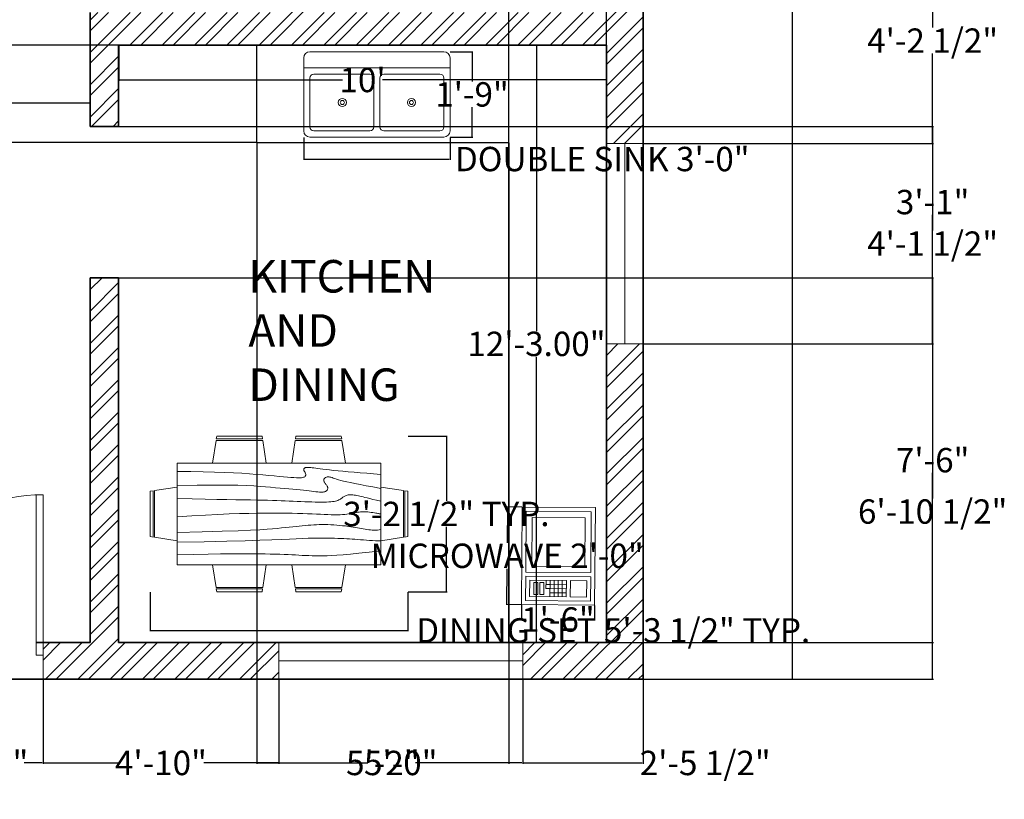
# Model space of a CAD drawing. Units: inches. Extents: x -20 to 887, y -143 to 410.
# Tile 2 of 5: x 139 to 381, y -11 to 180. Entities that reach past the tile are written whole.
import ezdxf

# ---------------------------------------------------------------- set-up
doc = ezdxf.new("R2010")
doc.units = ezdxf.units.IN
doc.header["$MEASUREMENT"] = 0
for name, color, linetype, lineweight in [('A-ANNO-DIMS', 2, 'Continuous', 18), ('A-AREA-IDEN', 7, 'Continuous', 25), ('A-DOOR', 3, 'Continuous', 18), ('A-EQPM', 9, 'Continuous', 18), ('A-FLOR-CASE', 9, 'Continuous', 25), ('A-FLOR-FIXT', 9, 'Continuous', 18), ('A-FURN', 8, 'Continuous', 18), ('A-GLAZ', 4, 'Continuous', 18), ('A-WALL', 7, 'Continuous', 35), ('A-WALL-PATT', 8, 'Continuous', 13)]:
    doc.layers.add(name, color=color, linetype=linetype, lineweight=lineweight)
doc.styles.get("Standard").update_dxf_attribs({"font": 'arial.ttf'})
doc.dimstyles.get("Standard").update_dxf_attribs({"dimtxt": 6, "dimasz": 0.18, "dimexe": 0.18, "dimexo": 0.0625, "dimgap": 0.09, "dimtad": 0, "dimtih": 1, "dimtoh": 1, "dimzin": 0, "dimdsep": 46, "dimlunit": 3, "dimtxsty": 'Standard', "dimcen": 0.09, "dimadec": 0, "dimazin": 0, "dimtfac": 1, "dimtofl": 0, "dimtmove": 0, "dimatfit": 3, "dimfxl": 1, "dimtolj": 1, "dimtzin": 0, "dimarcsym": 0})

# ---------------------------------------------------------------- blocks, each defined once
blk = doc.blocks.new('*U2')
for p, q in [((0, 0), (0, -6)), ((40, 0), (40, -6))]:
    blk.add_line(p, q)
blk.add_lwpolyline([(0, 0), (0, 40), (1.75, 40), (1.75, 0)], close=True)
blk.add_arc((0, 0), 40, 0, 90)
blk = doc.blocks.new('Microwave')
for p, q in [((18, 10), (22, 10)), ((19, 7), (19, 11)), ((20, 11), (20, 7)), ((21, 7), (21, 11)), ((22, 9), (18, 9)), ((18, 8), (22, 8)), ((22, 7), (18, 7)), ((20, 6), (18, 6)), ((19, 6), (19, 7)), ((20, 7), (20, 6))]:
    blk.add_line(p, q)
for points in [[(0, 0), (0, 18), (24, 18), (24, 0)], [(1, 1), (1, 17), (16, 17), (16, 1)], [(17, 1), (17, 17), (23, 17), (23, 1)], [(2.5, 2.5), (2.5, 15.5), (14.5, 15.5), (14.5, 2.5)], [(18, 12), (18, 16), (22, 16), (22, 12)], [(18, 2), (18, 11), (22, 11), (22, 2)], [(18.5, 4.5), (18.5, 5.5), (21.5, 5.5), (21.5, 4.5)], [(18.5, 3), (18.5, 4), (21.5, 4), (21.5, 3)]]:
    blk.add_lwpolyline(points, close=True)
blk = doc.blocks.new('Sink-double - 36 in top')
for p, q in [((-18, -4), (18, -4)), ((-0.75, -18.5), (-0.75, -6.5)), ((0.75, -6.5), (0.75, -18.5))]:
    blk.add_line(p, q)
for points in [[(-16.5, 0), (16.5, 0)], [(-18, -19.5), (-18, -1.5)], [(18, -1.5), (18, -19.5)], [(-16.5, -18.5), (-16.5, -6.5)], [(-15.5, -5.5), (-1.75, -5.5)], [(1.75, -5.5), (15.5, -5.5)], [(16.5, -6.5), (16.5, -18.5)], [(16.5, -21), (-16.5, -21)], [(-1.75, -19.5), (-15.5, -19.5)], [(15.5, -19.5), (1.75, -19.5)]]:
    blk.add_lwpolyline(points)
for centre, radius in [((-8.5, -12.5), 1), ((-8.5, -12.5), 0.5), ((8.5, -12.5), 1), ((8.5, -12.5), 0.5)]:
    blk.add_circle(centre, radius)
for centre, radius, start, end in [((-16.5, -1.5), 1.5, 90, 180), ((16.5, -1.5), 1.5, 0, 90), ((-15.5, -6.5), 1, 90, 180), ((-1.75, -6.5), 1, 0, 90), ((1.75, -6.5), 1, 90, 180), ((15.5, -6.5), 1, 0, 90), ((-15.5, -18.5), 1, 180, 270), ((-1.75, -18.5), 1, 270, 0), ((1.75, -18.5), 1, 180, 270), ((15.5, -18.5), 1, 270, 0), ((-16.5, -19.5), 1.5, 180, 270), ((16.5, -19.5), 1.5, 270, 0)]:
    blk.add_arc(centre, radius, start, end)
blk = doc.blocks.new('Dining Set - 36 x 72 in.')
for p, q in [((-22.2343, 26.00059), (-23.4847, 17.99762)), ((-22.2304, 26), (-5.7608, 26)), ((-22, 27.5), (-22.1562, 26.50042)), ((-5.8416, 26.5), (-22.1534, 26.5)), ((-22, 27.5), (-6, 27.5)), ((-5.8437, 26.49966), (-6, 27.5)), ((-4.5152, 17.99762), (-5.7655, 25.99926)), ((5.7657, 26.00059), (4.5153, 17.99762)), ((5.7696, 26), (22.2392, 26)), ((6, 27.5), (5.8438, 26.50042)), ((22.1584, 26.5), (5.8466, 26.5)), ((6, 27.5), (22, 27.5)), ((22.1563, 26.49966), (22, 27.5)), ((23.4848, 17.99762), (22.2345, 25.99926)), ((36, 18), (-36, 18)), ((-36, 18), (-36, -18)), ((36, -18), (36, 18)), ((-45.5, 8), (-44.5004, 8.15617)), ((-45.5, 8), (-45.5, -8)), ((-44.5, -8.15843), (-44.5, 8.15338)), ((-44.0006, 8.23428), (-35.9976, 9.48474)), ((-44, 8.23041), (-44, -8.23915)), ((44.0006, 8.23428), (35.9976, 9.48474)), ((44, 8.23041), (44, -8.23915)), ((44.5, -8.15843), (44.5, 8.15338)), ((45.5, 8), (44.5005, 8.15617)), ((45.5, 8), (45.5, -8)), ((-44.4997, -8.15631), (-45.5, -8)), ((-35.9976, -9.48476), (-43.9993, -8.2345)), ((35.9976, -9.48476), (43.9993, -8.2345)), ((44.4997, -8.15631), (45.5, -8)), ((-36, -18), (36, -18)), ((-22.2343, -26.0006), (-23.4847, -17.99762)), ((-4.5152, -17.99762), (-5.7655, -25.99928)), ((5.7657, -26.0006), (4.5153, -17.99762)), ((23.4848, -17.99762), (22.2345, -25.99928)), ((-22.2304, -26), (-5.7608, -26)), ((-22, -27.5), (-22.1562, -26.50044)), ((-5.8416, -26.5), (-22.1534, -26.5)), ((-22, -27.5), (-6, -27.5)), ((-5.8437, -26.49967), (-6, -27.5)), ((5.7696, -26), (22.2392, -26)), ((6, -27.5), (5.8438, -26.50044)), ((22.1584, -26.5), (5.8466, -26.5)), ((6, -27.5), (22, -27.5)), ((22.1563, -26.49967), (22, -27.5))]:
    blk.add_line(p, q)
for points in [[(-36, 15), (-31.1772, 14.97754), (-26.8079, 14.91406), (-22.8538, 14.81543), (-19.276, 14.6875), (-16.0362, 14.53613), (-13.0957, 14.36718), (-10.4159, 14.18652), (-7.9583, 14), (-5.6904, 13.81315), (-3.6035, 13.63021), (-1.6954, 13.45508), (0.0365, 13.29166), (1.5945, 13.14388), (2.9811, 13.01562), (4.1988, 12.9108), (5.25, 12.83333), (6.1393, 12.78613), (6.8802, 12.76823), (7.4883, 12.77767), (7.9792, 12.8125), (8.3685, 12.87077), (8.6719, 12.95052), (8.9049, 13.0498), (9.0833, 13.16666), (9.2205, 13.29899), (9.3216, 13.44401), (9.3895, 13.59879), (9.4271, 13.76041), (9.4373, 13.92594), (9.4232, 14.09245), (9.3875, 14.257), (9.3333, 14.41666), (9.2638, 14.56917), (9.1836, 14.71484), (9.0975, 14.85465), (9.0104, 14.98958), (8.9272, 15.1206), (8.8529, 15.2487), (8.7922, 15.37483), (8.75, 15.5), (8.7305, 15.62467), (8.7344, 15.74739), (8.7617, 15.86621), (8.8125, 15.97916), (8.8867, 16.08431), (8.9844, 16.17968), (9.1055, 16.26334), (9.25, 16.33333), (9.4189, 16.38802), (9.6172, 16.42708), (9.8506, 16.45052), (10.125, 16.45833), (10.4463, 16.45052), (10.8203, 16.42708), (11.2529, 16.38802), (11.75, 16.33333), (12.3184, 16.26318), (12.9694, 16.17838), (13.7151, 16.07991), (14.5677, 15.96875), (15.5395, 15.84586), (16.6426, 15.71224), (17.8893, 15.56884), (19.2917, 15.41666), (20.859, 15.25667), (22.5879, 15.08984), (24.4721, 14.91715), (26.5052, 14.73958), (28.6809, 14.5581), (30.9929, 14.3737), (33.4347, 14.18733), (36, 14)], [(-36, 10), (-28.9766, 10.14274), (-23.1725, 10.20442), (-18.4241, 10.19775), (-14.5677, 10.13541), (-11.4399, 10.03011), (-8.877, 9.89453), (-6.7154, 9.74137), (-4.7917, 9.58333), (-2.9698, 9.43082), (-1.2246, 9.28515), (0.4415, 9.14534), (2.026, 9.01041), (3.5266, 8.87939), (4.9408, 8.7513), (6.266, 8.62516), (7.5, 8.5), (8.6411, 8.37549), (9.6914, 8.2539), (10.6538, 8.13818), (11.5312, 8.03125), (12.3267, 7.93603), (13.043, 7.85547), (13.6831, 7.79248), (14.25, 7.75), (14.7471, 7.7303), (15.1797, 7.73307), (15.5537, 7.75732), (15.875, 7.80208), (16.1494, 7.86637), (16.3828, 7.94922), (16.5811, 8.04964), (16.75, 8.16666), (16.8944, 8.29915), (17.0143, 8.44531), (17.1089, 8.60319), (17.1771, 8.77083), (17.218, 8.94629), (17.2305, 9.1276), (17.2137, 9.31282), (17.1667, 9.5), (17.0895, 9.6875), (16.987, 9.875), (16.8649, 10.0625), (16.7292, 10.25), (16.5856, 10.4375), (16.4401, 10.625), (16.2985, 10.8125), (16.1667, 11), (16.05, 11.18733), (15.9518, 11.3737), (15.8752, 11.5581), (15.8229, 11.73958), (15.798, 11.91715), (15.8034, 12.08984), (15.842, 12.25667), (15.9167, 12.41666), (16.0295, 12.56836), (16.1784, 12.70833), (16.3605, 12.83268), (16.5729, 12.9375), (16.8127, 13.01888), (17.0768, 13.07291), (17.3625, 13.0957), (17.6667, 13.08333), (17.9894, 13.03312), (18.3418, 12.94726), (18.7382, 12.82918), (19.1927, 12.68229), (19.7195, 12.51001), (20.3327, 12.31575), (21.0465, 12.10294), (21.875, 11.875), (22.8357, 11.63354), (23.959, 11.37304), (25.2786, 11.08618), (26.8282, 10.76562), (28.6414, 10.40405), (30.752, 9.99414), (33.1936, 9.52856), (36, 9)], [(-36, 5.5), (-30.7157, 5.3348), (-26.069, 5.20963), (-21.9946, 5.11767), (-18.4271, 5.05208), (-15.3009, 5.00602), (-12.5508, 4.97265), (-10.1112, 4.94515), (-7.9167, 4.91666), (-5.909, 4.88167), (-4.0586, 4.83984), (-2.3429, 4.79215), (-0.7396, 4.73958), (0.7739, 4.6831), (2.22, 4.6237), (3.6213, 4.56233), (5, 4.5), (6.373, 4.43782), (7.7344, 4.3776), (9.0723, 4.32129), (10.375, 4.27083), (11.6309, 4.22819), (12.8281, 4.19531), (13.9551, 4.17415), (15, 4.16666), (15.954, 4.17448), (16.819, 4.19791), (17.6001, 4.23698), (18.3021, 4.29166), (18.9299, 4.36198), (19.4883, 4.44791), (19.9823, 4.54948), (20.4167, 4.66666), (20.7969, 4.79899), (21.1302, 4.94401), (21.4245, 5.09879), (21.6875, 5.26041), (21.9271, 5.42594), (22.1511, 5.59245), (22.3672, 5.757), (22.5834, 5.91666), (22.8065, 6.06868), (23.0404, 6.21093), (23.2879, 6.34147), (23.5521, 6.45833), (23.8358, 6.55957), (24.142, 6.64323), (24.4735, 6.70735), (24.8334, 6.75), (25.2235, 6.76969), (25.642, 6.76692), (26.0858, 6.74267), (26.5521, 6.69791), (27.0379, 6.63362), (27.5404, 6.55078), (28.0565, 6.45036), (28.5834, 6.33333), (29.1242, 6.19987), (29.7071, 6.04687), (30.3661, 5.87044), (31.1354, 5.66666), (32.0493, 5.43164), (33.142, 5.16146), (34.4475, 4.85221), (36, 4.5)], [(-36, -1), (-30.7915, -0.6591), (-26.0195, -0.38216), (-21.6519, -0.16284), (-17.6563, 0.00521), (-14.0005, 0.12833), (-10.6523, 0.21289), (-7.5796, 0.26522), (-4.75, 0.29166), (-2.134, 0.29793), (0.2878, 0.28711), (2.5317, 0.26163), (4.6146, 0.22396), (6.5529, 0.17651), (8.3633, 0.12174), (10.0623, 0.06209), (11.6667, 0), (13.1899, -0.06201), (14.6341, -0.1211), (15.9982, -0.17432), (17.2813, -0.21875), (18.4823, -0.25147), (19.6003, -0.26953), (20.6343, -0.27002), (21.5834, -0.25), (22.4481, -0.20768), (23.2357, -0.14584), (23.9549, -0.06836), (24.6146, 0.02083), (25.2235, 0.11784), (25.7904, 0.21875), (26.3241, 0.31966), (26.8334, 0.41666), (27.3265, 0.50618), (27.8099, 0.58593), (28.2894, 0.65397), (28.7709, 0.70833), (29.2601, 0.74707), (29.763, 0.76823), (30.2855, 0.76985), (30.8334, 0.75), (31.4088, 0.70784), (31.9994, 0.64713), (32.589, 0.57275), (33.1615, 0.48958), (33.7008, 0.4025), (34.1908, 0.3164), (34.6153, 0.23616), (34.9584, 0.16666), (35.2099, 0.11165), (35.3848, 0.07031), (35.504, 0.04069), (35.5886, 0.02083), (35.6594, 0.00879), (35.7377, 0.0026), (35.8442, 0.00032), (36, 0)], [(-36, -6.5), (-27.1843, -6.31267), (-20.084, -6.1263), (-14.469, -5.9419), (-10.1094, -5.76042), (-6.7752, -5.58285), (-4.2363, -5.41016), (-2.2629, -5.24333), (-0.625, -5.08334), (0.8708, -4.93099), (2.2715, -4.78646), (3.5872, -4.64974), (4.8281, -4.52084), (6.0046, -4.39974), (7.127, -4.28646), (8.2053, -4.18099), (9.25, -4.08334), (10.2705, -3.99382), (11.2734, -3.91407), (12.2647, -3.84603), (13.25, -3.79167), (14.2354, -3.75293), (15.2266, -3.73177), (16.2295, -3.73015), (17.25, -3.75), (18.2912, -3.79248), (19.3451, -3.85547), (20.4009, -3.93604), (21.4479, -4.03125), (22.4754, -4.13819), (23.4727, -4.25391), (24.4289, -4.37549), (25.3334, -4.5), (26.1785, -4.62492), (26.9694, -4.74935), (27.7145, -4.87281), (28.4219, -4.99479), (29.1, -5.11483), (29.7572, -5.23242), (30.4016, -5.34709), (31.0417, -5.45834), (31.6837, -5.56437), (32.3262, -5.65821), (32.9658, -5.73153), (33.599, -5.77604), (34.2224, -5.78345), (34.8327, -5.74545), (35.4264, -5.65373), (36, -5.5)], [(-36, -10), (-26.4022, -9.81299), (-18.4675, -9.62891), (-11.9839, -9.45069), (-6.7396, -9.28125), (-2.5226, -9.12354), (0.8789, -8.98047), (3.6769, -8.85498), (6.0833, -8.75), (8.2767, -8.66765), (10.3021, -8.60677), (12.1712, -8.56543), (13.8958, -8.54167), (15.4876, -8.53353), (16.9583, -8.53907), (18.3197, -8.55632), (19.5834, -8.58334), (20.7616, -8.61841), (21.8685, -8.66081), (22.9188, -8.71004), (23.9271, -8.76563), (24.9081, -8.82707), (25.8763, -8.89388), (26.8465, -8.96558), (27.8334, -9.04167), (28.8474, -9.12118), (29.8828, -9.20117), (30.93, -9.27824), (31.9792, -9.34896), (33.0205, -9.40991), (34.0443, -9.45768), (35.0407, -9.48885), (36, -9.5)], [(-36, -14.5), (-30.0881, -14.33513), (-25.0332, -14.21224), (-20.7312, -14.12647), (-17.0781, -14.07292), (-13.97, -14.04671), (-11.3027, -14.04297), (-8.9724, -14.05681), (-6.875, -14.08334), (-4.9224, -14.11833), (-3.0905, -14.16016), (-1.3709, -14.20785), (0.2448, -14.26042), (1.7647, -14.3169), (3.1973, -14.3763), (4.5507, -14.43767), (5.8333, -14.5), (7.0554, -14.5621), (8.235, -14.62175), (9.3922, -14.67652), (10.5469, -14.72396), (11.7192, -14.76164), (12.929, -14.78711), (14.1965, -14.79794), (15.5417, -14.79167), (16.9933, -14.76424), (18.6152, -14.70508), (20.4804, -14.60197), (22.6615, -14.44271), (25.2312, -14.21509), (28.2624, -13.9069), (31.8277, -13.50594), (36, -13)]]:
    blk.add_lwpolyline(points)
blk = doc.blocks.new('*D12')
at = {"layer": 'A-ANNO-DIMS', "color": 0, "lineweight": -2, "transparency": 16777216}
for p, q in [((25.42, 164.4), (25.42, 159.66)), ((156.42, 164.4), (156.42, 159.66)), ((25.6, 159.84), (72.65, 159.84)), ((156.24, 159.84), (109.19, 159.84))]:
    blk.add_line(p, q, dxfattribs=at)
at = {"layer": 'A-ANNO-DIMS', "color": 0, "transparency": 16777216}
for points in [[(25.6, 159.87), (25.6, 159.81), (25.42, 159.84)], [(156.24, 159.87), (156.24, 159.81), (156.42, 159.84)]]:
    blk.add_solid(points, dxfattribs=at)
at = {"layer": 'Defpoints', "color": 0, "transparency": 16777216}
for p in [(25.42, 164.46), (156.42, 164.46), (156.42, 159.84)]:
    blk.add_point(p, dxfattribs=at)
at = {"layer": 'A-ANNO-DIMS', "color": 0, "transparency": 16777216, "insert": (90.92, 159.84), "char_height": 6, "attachment_point": 5}
blk.add_mtext('\\A1;10\'-11.00"', dxfattribs=at)
blk = doc.blocks.new('*D13')
at = {"layer": 'A-ANNO-DIMS', "color": 0, "lineweight": -2, "transparency": 16777216}
for p, q in [((163.42, 174.07), (163.42, 165.37)), ((283.42, 174.07), (283.42, 165.37)), ((163.6, 165.55), (218.52, 165.55)), ((283.24, 165.55), (228.32, 165.55))]:
    blk.add_line(p, q, dxfattribs=at)
at = {"layer": 'A-ANNO-DIMS', "color": 0, "transparency": 16777216}
for points in [[(163.6, 165.58), (163.6, 165.52), (163.42, 165.55)], [(283.24, 165.58), (283.24, 165.52), (283.42, 165.55)]]:
    blk.add_solid(points, dxfattribs=at)
at = {"layer": 'Defpoints', "color": 0, "transparency": 16777216}
for p in [(163.42, 174.13), (283.42, 174.13), (283.42, 165.55)]:
    blk.add_point(p, dxfattribs=at)
at = {"layer": 'A-ANNO-DIMS', "color": 0, "transparency": 16777216, "insert": (223.42, 165.55), "char_height": 6, "attachment_point": 5}
blk.add_mtext("\\A1;10'", dxfattribs=at)
blk = doc.blocks.new('*D14')
at = {"layer": 'A-ANNO-DIMS', "color": 0, "lineweight": -2, "transparency": 16777216}
for p, q in [((283.35, 174.13), (266.02, 174.13)), ((266.2, 173.95), (266.2, 103.79)), ((266.2, 27.31), (266.2, 97.48)), ((283.35, 27.13), (266.02, 27.13))]:
    blk.add_line(p, q, dxfattribs=at)
at = {"layer": 'A-ANNO-DIMS', "color": 0, "transparency": 16777216}
for points in [[(266.17, 173.95), (266.23, 173.95), (266.2, 174.13)], [(266.17, 27.31), (266.23, 27.31), (266.2, 27.13)]]:
    blk.add_solid(points, dxfattribs=at)
at = {"layer": 'Defpoints', "color": 0, "transparency": 16777216}
for p in [(266.2, 174.13), (283.42, 174.13), (283.42, 27.13)]:
    blk.add_point(p, dxfattribs=at)
at = {"layer": 'A-ANNO-DIMS', "color": 0, "transparency": 16777216, "insert": (266.2, 100.63), "char_height": 6, "attachment_point": 5}
blk.add_mtext('\\A1;12\'-3.00"', dxfattribs=at)
blk = doc.blocks.new('*D22')
at = {"layer": 'A-ANNO-DIMS', "color": 0, "lineweight": -2, "transparency": 16777216}
for p, q in [((292.48, 378.13), (329.35, 378.13)), ((329.17, 377.95), (329.17, 201.29)), ((329.17, 18.31), (329.17, 194.98)), ((292.48, 18.13), (329.35, 18.13))]:
    blk.add_line(p, q, dxfattribs=at)
at = {"layer": 'A-ANNO-DIMS', "color": 0, "transparency": 16777216}
for points in [[(329.14, 377.95), (329.2, 377.95), (329.17, 378.13)], [(329.14, 18.31), (329.2, 18.31), (329.17, 18.13)]]:
    blk.add_solid(points, dxfattribs=at)
at = {"layer": 'Defpoints', "color": 0, "transparency": 16777216}
for p in [(292.42, 378.13), (292.42, 18.13), (329.17, 18.13)]:
    blk.add_point(p, dxfattribs=at)
at = {"layer": 'A-ANNO-DIMS', "color": 0, "transparency": 16777216, "insert": (329.17, 198.13), "char_height": 6, "attachment_point": 5}
blk.add_mtext("\\A1;30'", dxfattribs=at)
blk = doc.blocks.new('*D47')
at = {"layer": 'A-ANNO-DIMS', "color": 0, "lineweight": -2, "transparency": 16777216}
for p, q in [((171.19, 39.58), (171.19, 29.96)), ((234.54, 39.58), (234.54, 29.96)), ((171.37, 30.14), (234.36, 30.14)), ((234.54, 30.14), (234.72, 30.14))]:
    blk.add_line(p, q, dxfattribs=at)
at = {"layer": 'A-ANNO-DIMS', "color": 0, "transparency": 16777216}
for points in [[(171.37, 30.17), (171.37, 30.11), (171.19, 30.14)], [(234.36, 30.17), (234.36, 30.11), (234.54, 30.14)]]:
    blk.add_solid(points, dxfattribs=at)
at = {"layer": 'Defpoints', "color": 0, "transparency": 16777216}
for p in [(171.19, 39.64), (234.54, 39.64), (234.54, 30.14)]:
    blk.add_point(p, dxfattribs=at)
at = {"layer": 'A-ANNO-DIMS', "color": 0, "transparency": 16777216, "insert": (285.08, 30.14), "char_height": 6, "attachment_point": 5}
blk.add_mtext('\\A1;DINING SET 5\'-3 1/2" TYP.', dxfattribs=at)
blk = doc.blocks.new('*D48')
at = {"layer": 'A-ANNO-DIMS', "color": 0, "lineweight": -2, "transparency": 16777216}
for p, q in [((234.6, 77.93), (244.22, 77.93)), ((244.04, 77.75), (244.04, 61.98)), ((244.04, 39.82), (244.04, 55.59)), ((234.6, 39.64), (244.22, 39.64))]:
    blk.add_line(p, q, dxfattribs=at)
at = {"layer": 'A-ANNO-DIMS', "color": 0, "transparency": 16777216}
for points in [[(244.01, 77.75), (244.07, 77.75), (244.04, 77.93)], [(244.01, 39.82), (244.07, 39.82), (244.04, 39.64)]]:
    blk.add_solid(points, dxfattribs=at)
at = {"layer": 'Defpoints', "color": 0, "transparency": 16777216}
for p in [(234.54, 77.93), (244.04, 77.93), (234.54, 39.64)]:
    blk.add_point(p, dxfattribs=at)
at = {"layer": 'A-ANNO-DIMS', "color": 0, "transparency": 16777216, "insert": (244.04, 58.79), "char_height": 6, "attachment_point": 5}
blk.add_mtext('\\A1;3\'-2 1/2" TYP.', dxfattribs=at)
blk = doc.blocks.new('*D49')
at = {"layer": 'A-ANNO-DIMS', "color": 0, "lineweight": -2, "transparency": 16777216}
for p, q in [((262.63, 60.47), (258.91, 60.5)), ((259.09, 60.32), (259.02, 51.7)), ((258.91, 36.68), (258.97, 45.31)), ((262.45, 36.47), (258.73, 36.5))]:
    blk.add_line(p, q, dxfattribs=at)
at = {"layer": 'A-ANNO-DIMS', "color": 0, "transparency": 16777216}
for points in [[(259.06, 60.32), (259.12, 60.32), (259.09, 60.5)], [(258.88, 36.68), (258.94, 36.68), (258.91, 36.5)]]:
    blk.add_solid(points, dxfattribs=at)
at = {"layer": 'Defpoints', "color": 0, "transparency": 16777216}
for p in [(262.69, 60.47), (258.91, 36.5), (262.51, 36.47)]:
    blk.add_point(p, dxfattribs=at)
at = {"layer": 'A-ANNO-DIMS', "color": 0, "transparency": 16777216, "insert": (259, 48.5), "char_height": 6, "attachment_point": 5}
blk.add_mtext('\\A1;MICROWAVE 2\'-0"', dxfattribs=at)
blk = doc.blocks.new('*D50')
at = {"layer": 'A-ANNO-DIMS', "color": 0, "lineweight": -2, "transparency": 16777216}
for p, q in [((262.51, 36.41), (262.48, 32.69)), ((280.51, 36.27), (280.48, 32.56)), ((262.66, 32.87), (263.7, 32.87)), ((280.3, 32.74), (279.26, 32.75))]:
    blk.add_line(p, q, dxfattribs=at)
at = {"layer": 'A-ANNO-DIMS', "color": 0, "transparency": 16777216}
for points in [[(262.66, 32.9), (262.66, 32.84), (262.48, 32.87)], [(280.3, 32.77), (280.3, 32.71), (280.48, 32.74)]]:
    blk.add_solid(points, dxfattribs=at)
at = {"layer": 'Defpoints', "color": 0, "transparency": 16777216}
for p in [(262.51, 36.47), (280.51, 36.34), (280.48, 32.74)]:
    blk.add_point(p, dxfattribs=at)
at = {"layer": 'A-ANNO-DIMS', "color": 0, "transparency": 16777216, "insert": (271.48, 32.81), "char_height": 6, "attachment_point": 5}
blk.add_mtext('\\A1;1\'-6"', dxfattribs=at)
blk = doc.blocks.new('*D51')
at = {"layer": 'A-ANNO-DIMS', "color": 0, "lineweight": -2, "transparency": 16777216}
for p, q in [((208.94, 151.44), (208.94, 145.92)), ((244.94, 151.44), (244.94, 145.92)), ((209.12, 146.1), (244.76, 146.1)), ((244.94, 146.1), (245.12, 146.1))]:
    blk.add_line(p, q, dxfattribs=at)
at = {"layer": 'A-ANNO-DIMS', "color": 0, "transparency": 16777216}
for points in [[(209.12, 146.13), (209.12, 146.07), (208.94, 146.1)], [(244.76, 146.13), (244.76, 146.07), (244.94, 146.1)]]:
    blk.add_solid(points, dxfattribs=at)
at = {"layer": 'Defpoints', "color": 0, "transparency": 16777216}
for p in [(208.94, 151.5), (244.94, 151.5), (244.94, 146.1)]:
    blk.add_point(p, dxfattribs=at)
at = {"layer": 'A-ANNO-DIMS', "color": 0, "transparency": 16777216, "insert": (282.38, 146.1), "char_height": 6, "attachment_point": 5}
blk.add_mtext('\\A1;DOUBLE SINK 3\'-0"', dxfattribs=at)
blk = doc.blocks.new('*D52')
at = {"layer": 'A-ANNO-DIMS', "color": 0, "lineweight": -2, "transparency": 16777216}
for p, q in [((245, 172.5), (250.52, 172.5)), ((250.34, 172.32), (250.34, 165.16)), ((250.34, 151.68), (250.34, 158.85)), ((245, 151.5), (250.52, 151.5))]:
    blk.add_line(p, q, dxfattribs=at)
at = {"layer": 'A-ANNO-DIMS', "color": 0, "transparency": 16777216}
for points in [[(250.31, 172.32), (250.37, 172.32), (250.34, 172.5)], [(250.31, 151.68), (250.37, 151.68), (250.34, 151.5)]]:
    blk.add_solid(points, dxfattribs=at)
at = {"layer": 'Defpoints', "color": 0, "transparency": 16777216}
for p in [(244.94, 172.5), (250.34, 172.5), (244.94, 151.5)]:
    blk.add_point(p, dxfattribs=at)
at = {"layer": 'A-ANNO-DIMS', "color": 0, "transparency": 16777216, "insert": (250.34, 162), "char_height": 6, "attachment_point": 5}
blk.add_mtext('\\A1;1\'-9"', dxfattribs=at)
blk = doc.blocks.new('*D54')
at = {"layer": 'A-ANNO-DIMS', "color": 0, "lineweight": -2, "transparency": 16777216}
for p, q in [((105.35, 18.07), (105.35, -2.65)), ((144.81, 18.07), (144.81, -2.65)), ((105.53, -2.47), (110.03, -2.47)), ((144.63, -2.47), (140.13, -2.47))]:
    blk.add_line(p, q, dxfattribs=at)
at = {"layer": 'A-ANNO-DIMS', "color": 0, "transparency": 16777216}
for points in [[(105.53, -2.44), (105.53, -2.5), (105.35, -2.47)], [(144.63, -2.44), (144.63, -2.5), (144.81, -2.47)]]:
    blk.add_solid(points, dxfattribs=at)
at = {"layer": 'Defpoints', "color": 0, "transparency": 16777216}
for p in [(105.35, 18.13), (144.81, 18.13), (144.81, -2.47)]:
    blk.add_point(p, dxfattribs=at)
at = {"layer": 'A-ANNO-DIMS', "color": 0, "transparency": 16777216, "insert": (125.08, -2.47), "char_height": 6, "attachment_point": 5}
blk.add_mtext('\\A1;3\'-3 1/2"', dxfattribs=at)
blk = doc.blocks.new('*D55')
at = {"layer": 'A-ANNO-DIMS', "color": 0, "lineweight": -2, "transparency": 16777216}
for p, q in [((144.81, 18.07), (144.81, -2.65)), ((202.81, 18.07), (202.81, -2.65)), ((144.99, -2.47), (163.3, -2.47)), ((202.63, -2.47), (184.33, -2.47))]:
    blk.add_line(p, q, dxfattribs=at)
at = {"layer": 'A-ANNO-DIMS', "color": 0, "transparency": 16777216}
for points in [[(144.99, -2.44), (144.99, -2.5), (144.81, -2.47)], [(202.63, -2.44), (202.63, -2.5), (202.81, -2.47)]]:
    blk.add_solid(points, dxfattribs=at)
at = {"layer": 'Defpoints', "color": 0, "transparency": 16777216}
for p in [(144.81, 18.13), (202.81, 18.13), (202.81, -2.47)]:
    blk.add_point(p, dxfattribs=at)
at = {"layer": 'A-ANNO-DIMS', "color": 0, "transparency": 16777216, "insert": (173.81, -2.47), "char_height": 6, "attachment_point": 5}
blk.add_mtext('\\A1;4\'-10"', dxfattribs=at)
blk = doc.blocks.new('*D56')
at = {"layer": 'A-ANNO-DIMS', "color": 0, "lineweight": -2, "transparency": 16777216}
for p, q in [((202.81, 18.07), (202.81, -2.65)), ((262.81, 18.07), (262.81, -2.65)), ((202.99, -2.47), (224.75, -2.47)), ((262.63, -2.47), (240.88, -2.47))]:
    blk.add_line(p, q, dxfattribs=at)
at = {"layer": 'A-ANNO-DIMS', "color": 0, "transparency": 16777216}
for points in [[(202.99, -2.44), (202.99, -2.5), (202.81, -2.47)], [(262.63, -2.44), (262.63, -2.5), (262.81, -2.47)]]:
    blk.add_solid(points, dxfattribs=at)
at = {"layer": 'Defpoints', "color": 0, "transparency": 16777216}
for p in [(202.81, 18.13), (262.81, 18.13), (262.81, -2.47)]:
    blk.add_point(p, dxfattribs=at)
at = {"layer": 'A-ANNO-DIMS', "color": 0, "transparency": 16777216, "insert": (232.81, -2.47), "char_height": 6, "attachment_point": 5}
blk.add_mtext('\\A1;5\'-0"', dxfattribs=at)
blk = doc.blocks.new('*D57')
at = {"layer": 'A-ANNO-DIMS', "color": 0, "lineweight": -2, "transparency": 16777216}
for p, q in [((262.81, 18.07), (262.81, -2.65)), ((292.42, 18.07), (292.42, -2.65)), ((262.99, -2.47), (292.24, -2.47)), ((292.42, -2.47), (292.6, -2.47))]:
    blk.add_line(p, q, dxfattribs=at)
at = {"layer": 'A-ANNO-DIMS', "color": 0, "transparency": 16777216}
for points in [[(262.99, -2.44), (262.99, -2.5), (262.81, -2.47)], [(292.24, -2.44), (292.24, -2.5), (292.42, -2.47)]]:
    blk.add_solid(points, dxfattribs=at)
at = {"layer": 'Defpoints', "color": 0, "transparency": 16777216}
for p in [(262.81, 18.13), (292.42, 18.13), (292.42, -2.47)]:
    blk.add_point(p, dxfattribs=at)
at = {"layer": 'A-ANNO-DIMS', "color": 0, "transparency": 16777216, "insert": (307.7, -2.47), "char_height": 6, "attachment_point": 5}
blk.add_mtext('\\A1;2\'-5 1/2"', dxfattribs=at)
blk = doc.blocks.new('*D61')
at = {"layer": 'A-ANNO-DIMS', "color": 0, "lineweight": -2, "transparency": 16777216}
for p, q in [((292.48, 100.63), (363.84, 100.63)), ((363.66, 100.45), (363.66, 62.58)), ((363.66, 18.31), (363.66, 56.19)), ((292.48, 18.13), (363.84, 18.13))]:
    blk.add_line(p, q, dxfattribs=at)
at = {"layer": 'A-ANNO-DIMS', "color": 0, "transparency": 16777216}
for points in [[(363.63, 100.45), (363.69, 100.45), (363.66, 100.63)], [(363.63, 18.31), (363.69, 18.31), (363.66, 18.13)]]:
    blk.add_solid(points, dxfattribs=at)
at = {"layer": 'Defpoints', "color": 0, "transparency": 16777216}
for p in [(292.42, 100.63), (363.66, 100.63), (292.42, 18.13)]:
    blk.add_point(p, dxfattribs=at)
at = {"layer": 'A-ANNO-DIMS', "color": 0, "transparency": 16777216, "insert": (363.66, 59.38), "char_height": 6, "attachment_point": 5}
blk.add_mtext('\\A1;6\'-10 1/2"', dxfattribs=at)
blk = doc.blocks.new('*D62')
at = {"layer": 'A-ANNO-DIMS', "color": 0, "lineweight": -2, "transparency": 16777216}
for p, q in [((292.48, 149.94), (363.84, 149.94)), ((363.66, 149.76), (363.66, 128.48)), ((363.66, 100.81), (363.66, 122.09)), ((292.48, 100.63), (363.84, 100.63))]:
    blk.add_line(p, q, dxfattribs=at)
at = {"layer": 'A-ANNO-DIMS', "color": 0, "transparency": 16777216}
for points in [[(363.63, 149.76), (363.69, 149.76), (363.66, 149.94)], [(363.63, 100.81), (363.69, 100.81), (363.66, 100.63)]]:
    blk.add_solid(points, dxfattribs=at)
at = {"layer": 'Defpoints', "color": 0, "transparency": 16777216}
for p in [(292.42, 149.94), (363.66, 149.94), (292.42, 100.63)]:
    blk.add_point(p, dxfattribs=at)
at = {"layer": 'A-ANNO-DIMS', "color": 0, "transparency": 16777216, "insert": (363.66, 125.29), "char_height": 6, "attachment_point": 5}
blk.add_mtext('\\A1;4\'-1 1/2"', dxfattribs=at)
blk = doc.blocks.new('*D63')
at = {"layer": 'A-ANNO-DIMS', "color": 0, "lineweight": -2, "transparency": 16777216}
for p, q in [((292.48, 200.53), (363.84, 200.53)), ((363.66, 200.35), (363.66, 178.43)), ((363.66, 150.12), (363.66, 172.04)), ((292.48, 149.94), (363.84, 149.94))]:
    blk.add_line(p, q, dxfattribs=at)
at = {"layer": 'A-ANNO-DIMS', "color": 0, "transparency": 16777216}
for points in [[(363.63, 200.35), (363.69, 200.35), (363.66, 200.53)], [(363.63, 150.12), (363.69, 150.12), (363.66, 149.94)]]:
    blk.add_solid(points, dxfattribs=at)
at = {"layer": 'Defpoints', "color": 0, "transparency": 16777216}
for p in [(292.42, 200.53), (363.66, 200.53), (292.42, 149.94)]:
    blk.add_point(p, dxfattribs=at)
at = {"layer": 'A-ANNO-DIMS', "color": 0, "transparency": 16777216, "insert": (363.66, 175.23), "char_height": 6, "attachment_point": 5}
blk.add_mtext('\\A1;4\'-2 1/2"', dxfattribs=at)
blk = doc.blocks.new('*D66')
at = {"layer": 'A-ANNO-DIMS', "color": 0, "lineweight": -2, "transparency": 16777216}
for p, q in [((163.48, 154.1), (363.84, 154.1)), ((363.66, 153.92), (363.66, 138.66)), ((363.66, 117.09), (363.66, 132.35)), ((163.48, 116.91), (363.84, 116.91))]:
    blk.add_line(p, q, dxfattribs=at)
at = {"layer": 'A-ANNO-DIMS', "color": 0, "transparency": 16777216}
for points in [[(363.63, 153.92), (363.69, 153.92), (363.66, 154.1)], [(363.63, 117.09), (363.69, 117.09), (363.66, 116.91)]]:
    blk.add_solid(points, dxfattribs=at)
at = {"layer": 'Defpoints', "color": 0, "transparency": 16777216}
for p in [(163.42, 154.1), (163.42, 116.91), (363.66, 116.91)]:
    blk.add_point(p, dxfattribs=at)
at = {"layer": 'A-ANNO-DIMS', "color": 0, "transparency": 16777216, "insert": (363.66, 135.51), "char_height": 6, "attachment_point": 5}
blk.add_mtext('\\A1;3\'-1"', dxfattribs=at)
blk = doc.blocks.new('*D67')
at = {"layer": 'A-ANNO-DIMS', "color": 0, "lineweight": -2, "transparency": 16777216}
for p, q in [((163.48, 116.91), (363.84, 116.91)), ((363.66, 116.73), (363.66, 75.18)), ((363.66, 27.31), (363.66, 68.87)), ((163.48, 27.13), (363.84, 27.13))]:
    blk.add_line(p, q, dxfattribs=at)
at = {"layer": 'A-ANNO-DIMS', "color": 0, "transparency": 16777216}
for points in [[(363.63, 116.73), (363.69, 116.73), (363.66, 116.91)], [(363.63, 27.31), (363.69, 27.31), (363.66, 27.13)]]:
    blk.add_solid(points, dxfattribs=at)
at = {"layer": 'Defpoints', "color": 0, "transparency": 16777216}
for p in [(163.42, 116.91), (163.42, 27.13), (363.66, 27.13)]:
    blk.add_point(p, dxfattribs=at)
at = {"layer": 'A-ANNO-DIMS', "color": 0, "transparency": 16777216, "insert": (363.66, 72.02), "char_height": 6, "attachment_point": 5}
blk.add_mtext('\\A1;7\'-6"', dxfattribs=at)
blk = doc.blocks.new('*D68')
at = {"layer": 'A-ANNO-DIMS', "color": 0, "lineweight": -2, "transparency": 16777216}
for p, q in [((197.32, 174.13), (-4.36, 174.13)), ((-4.18, 173.95), (-4.18, 165.29)), ((-4.18, 150.31), (-4.18, 158.98)), ((197.32, 150.13), (-4.36, 150.13))]:
    blk.add_line(p, q, dxfattribs=at)
at = {"layer": 'A-ANNO-DIMS', "color": 0, "transparency": 16777216}
for points in [[(-4.21, 173.95), (-4.15, 173.95), (-4.18, 174.13)], [(-4.21, 150.31), (-4.15, 150.31), (-4.18, 150.13)]]:
    blk.add_solid(points, dxfattribs=at)
at = {"layer": 'Defpoints', "color": 0, "transparency": 16777216}
for p in [(197.38, 174.13), (-4.18, 150.13), (197.38, 150.13)]:
    blk.add_point(p, dxfattribs=at)
at = {"layer": 'A-ANNO-DIMS', "color": 0, "transparency": 16777216, "insert": (-4.18, 162.13), "char_height": 6, "attachment_point": 5}
blk.add_mtext('\\A1;2\'-0"', dxfattribs=at)
blk = doc.blocks.new('*D69')
at = {"layer": 'A-ANNO-DIMS', "color": 0, "lineweight": -2, "transparency": 16777216}
for p, q in [((197.38, 150.07), (197.38, -2.65)), ((259.42, 150.07), (259.42, -2.65)), ((197.56, -2.47), (220.33, -2.47)), ((259.24, -2.47), (236.46, -2.47))]:
    blk.add_line(p, q, dxfattribs=at)
at = {"layer": 'A-ANNO-DIMS', "color": 0, "transparency": 16777216}
for points in [[(197.56, -2.44), (197.56, -2.5), (197.38, -2.47)], [(259.24, -2.44), (259.24, -2.5), (259.42, -2.47)]]:
    blk.add_solid(points, dxfattribs=at)
at = {"layer": 'Defpoints', "color": 0, "transparency": 16777216}
for p in [(197.38, 150.13), (259.42, 150.13), (259.42, -2.47)]:
    blk.add_point(p, dxfattribs=at)
at = {"layer": 'A-ANNO-DIMS', "color": 0, "transparency": 16777216, "insert": (228.4, -2.47), "char_height": 6, "attachment_point": 5}
blk.add_mtext('\\A1;5\'-2"', dxfattribs=at)
blk = doc.blocks.new('*D70')
at = {"layer": 'A-ANNO-DIMS', "color": 0, "lineweight": -2, "transparency": 16777216}
for p, q in [((259.42, 27.2), (259.42, 398.91)), ((259.6, 398.73), (263.3, 398.73)), ((283.24, 398.73), (279.53, 398.73)), ((283.42, 27.2), (283.42, 398.91))]:
    blk.add_line(p, q, dxfattribs=at)
at = {"layer": 'A-ANNO-DIMS', "color": 0, "transparency": 16777216}
for points in [[(259.6, 398.76), (259.6, 398.7), (259.42, 398.73)], [(283.24, 398.76), (283.24, 398.7), (283.42, 398.73)]]:
    blk.add_solid(points, dxfattribs=at)
at = {"layer": 'Defpoints', "color": 0, "transparency": 16777216}
for p in [(283.42, 398.73), (259.42, 27.13), (283.42, 27.13)]:
    blk.add_point(p, dxfattribs=at)
at = {"layer": 'A-ANNO-DIMS', "color": 0, "transparency": 16777216, "insert": (271.42, 398.73), "char_height": 6, "attachment_point": 5}
blk.add_mtext('\\A1;2\'-0"', dxfattribs=at)

msp = doc.modelspace()

# ---------------------------------------------------------------- hatches: boundary and pattern name
at = {"layer": 'A-WALL-PATT'}
h = msp.add_hatch(dxfattribs=at)
h.set_pattern_fill('ANSI32', color=256, scale=15)
h.paths.add_polyline_path([(292.417, 200.529), (283.417, 200.529), (283.417, 182.135), (211.417, 182.135), (211.417, 210.612, -0.0394206), (207.838, 210.33), (204.417, 210.33), (204.417, 182.135), (156.417, 182.135), (156.417, 154.102), (163.417, 154.102), (163.417, 174.135), (283.417, 174.135), (283.417, 149.94), (292.417, 149.94)])
h = msp.add_hatch(dxfattribs=at)
h.set_pattern_fill('ANSI32', color=256, scale=15)
h.paths.add_polyline_path([(202.813, 27.135), (163.417, 27.135), (163.417, 116.909), (156.417, 116.909), (156.417, 27.135), (144.81, 27.135), (144.81, 24.054), (144.81, 18.135), (202.813, 18.135)])
h = msp.add_hatch(dxfattribs=at)
h.set_pattern_fill('ANSI32', color=256, scale=15)
h.paths.add_polyline_path([(292.417, 100.635), (283.417, 100.635), (283.417, 27.135), (262.813, 27.135), (262.813, 18.135), (292.417, 18.135)])

# ---------------------------------------------------------------- linework, layer by layer
at = {"layer": 'A-FLOR-CASE'}
msp.add_line((197.379, 150.135), (197.379, 174.135), dxfattribs=at)
for points in [[(197.379, 150.135), (259.417, 150.135)], [(259.417, 27.135), (259.417, 150.135)]]:
    msp.add_lwpolyline(points, dxfattribs=at)
at = {"layer": 'A-GLAZ'}
for p, q in [((283.417, 149.94), (292.417, 149.94)), ((287.917, 149.94), (287.917, 100.635)), ((283.417, 100.635), (292.417, 100.635)), ((202.813, 27.135), (202.813, 18.135)), ((262.813, 27.135), (262.813, 18.135)), ((202.813, 22.635), (262.813, 22.635))]:
    msp.add_line(p, q, dxfattribs=at)
at = {"layer": 'A-WALL'}
for p, q in [((156.417, 154.102), (163.417, 154.102)), ((156.417, 116.909), (163.417, 116.909))]:
    msp.add_line(p, q, dxfattribs=at)
msp.add_lwpolyline([(16.417, 18.135), (292.417, 18.135), (292.417, 378.135), (16.417, 378.135)], close=True, dxfattribs=at)
for points in [[(156.417, 182.135), (156.417, 154.102)], [(163.417, 174.135), (283.417, 174.135)], [(163.417, 154.102), (163.417, 174.135)], [(283.417, 27.135), (283.417, 174.135)], [(156.417, 116.909), (156.417, 27.135)], [(163.417, 27.135), (163.417, 116.909)], [(143.084, 27.135), (156.417, 27.135)], [(163.417, 27.135), (283.417, 27.135)]]:
    msp.add_lwpolyline(points, dxfattribs=at)

# ---------------------------------------------------------------- block references
at = {"layer": 'A-DOOR', "xscale": -0.9865145828543779, "yscale": 0.9865145828543779, "zscale": 0.9865145828543779}
msp.add_blockref('*U2', (144.81, 24.054), dxfattribs=at)
at = {"layer": 'A-EQPM', "rotation": 269.5621064421589}
msp.add_blockref('Microwave', (262.691, 60.474), dxfattribs=at)
at = {"layer": 'A-FLOR-FIXT'}
msp.add_blockref('Sink-double - 36 in top', (226.941, 172.503), dxfattribs=at)
at = {"layer": 'A-FURN', "xscale": 0.6961336996175513, "yscale": 0.6961336996175513, "zscale": 0.6961336996175513}
msp.add_blockref('Dining Set - 36 x 72 in.', (202.863, 58.786), dxfattribs=at)

# ---------------------------------------------------------------- texts
at = {"layer": 'A-AREA-IDEN', "insert": (195.321, 121.258), "char_height": 8, "attachment_point": 1}
msp.add_mtext_dynamic_manual_height_columns('KITCHEN AND DINING ', width=50.36765, gutter_width=1, heights=[0], dxfattribs=at)

# ---------------------------------------------------------------- dimensions: what is measured, and where the dimension line sits
at = {"layer": 'A-ANNO-DIMS'}
for base, p1, p2, override, picture, middle in [((283.417, 398.735), (259.417, 27.135), (283.417, 27.135), {"dimdec": 1, "dimlfac": 1, "dimrnd": 0, "dimzin": 1, "dimdsep": 46, "dimlunit": 4, "dimfrac": 2}, '*D70', (271.417, 398.735)), ((283.417, 165.549), (163.417, 174.135), (283.417, 174.135), {"dimclrd": 0, "dimclre": 0, "dimclrt": 0}, '*D13', (223.417, 165.549)), ((156.417, 159.836), (25.417, 164.461), (156.417, 164.461), {"dimclrd": 0, "dimclre": 0, "dimclrt": 0}, '*D12', (90.917, 159.836)), ((259.417, -2.465), (197.379, 150.135), (259.417, 150.135), {"dimdec": 1, "dimlfac": 1, "dimrnd": 0, "dimzin": 1, "dimdsep": 46, "dimlunit": 4, "dimfrac": 2}, '*D69', (228.398, -2.465)), ((144.81, -2.465), (105.35, 18.135), (144.81, 18.135), {"dimdec": 1, "dimlfac": 1, "dimrnd": 0, "dimzin": 1, "dimdsep": 46, "dimlunit": 4, "dimfrac": 2}, '*D54', (125.08, -2.465)), ((202.813, -2.465), (144.81, 18.135), (202.813, 18.135), {"dimdec": 1, "dimlfac": 1, "dimrnd": 0, "dimzin": 1, "dimdsep": 46, "dimlunit": 4, "dimfrac": 2}, '*D55', (173.812, -2.465)), ((262.813, -2.465), (202.813, 18.135), (262.813, 18.135), {"dimdec": 1, "dimlfac": 1, "dimrnd": 0, "dimzin": 1, "dimdsep": 46, "dimlunit": 4, "dimfrac": 2}, '*D56', (232.813, -2.465)), ((292.417, -2.465), (262.813, 18.135), (292.417, 18.135), {"dimdec": 1, "dimlfac": 1, "dimrnd": 0, "dimzin": 1, "dimdsep": 46, "dimlunit": 4, "dimfrac": 2}, '*D57', (307.703, -2.465))]:
    dim = msp.add_linear_dim(base=base, p1=p1, p2=p2, dimstyle='Standard', override=override, dxfattribs=at)
    dim.commit()
    dim.dimension.update_dxf_attribs({"geometry": picture, "text_midpoint": middle})
for base, p1, p2, angle, override, picture, middle in [((329.167, 18.135), (292.417, 378.135), (292.417, 18.135), 90, {"dimclrd": 0, "dimclre": 0, "dimclrt": 0}, '*D22', (329.167, 198.135)), ((363.657, 200.529), (292.417, 149.94), (292.417, 200.529), 90, {"dimdec": 1, "dimlfac": 1, "dimrnd": 0, "dimzin": 1, "dimdsep": 46, "dimlunit": 4, "dimfrac": 2}, '*D63', (363.657, 175.234)), ((-4.183, 150.135), (197.379, 174.135), (197.379, 150.135), 90, {"dimdec": 1, "dimlfac": 1, "dimrnd": 0, "dimzin": 1, "dimdsep": 46, "dimlunit": 4, "dimfrac": 2}, '*D68', (-4.183, 162.135)), ((250.341, 172.503), (244.941, 151.503), (244.941, 172.503), 90, {"dimdec": 1, "dimlfac": 1, "dimrnd": 0, "dimzin": 1, "dimdsep": 46, "dimlunit": 4, "dimfrac": 2}, '*D52', (250.341, 162.003)), ((266.198, 174.135), (283.417, 27.135), (283.417, 174.135), 90, {"dimclrd": 0, "dimclre": 0, "dimclrt": 0}, '*D14', (266.198, 100.635)), ((363.657, 116.909), (163.417, 154.102), (163.417, 116.909), 90, {"dimdec": 1, "dimlfac": 1, "dimrnd": 0, "dimzin": 1, "dimdsep": 46, "dimlunit": 4, "dimfrac": 2}, '*D66', (363.657, 135.505)), ((363.657, 149.94), (292.417, 100.635), (292.417, 149.94), 90, {"dimdec": 1, "dimlfac": 1, "dimrnd": 0, "dimzin": 1, "dimdsep": 46, "dimlunit": 4, "dimfrac": 2}, '*D62', (363.657, 125.287)), ((363.657, 27.135), (163.417, 116.909), (163.417, 27.135), 90, {"dimdec": 1, "dimlfac": 1, "dimrnd": 0, "dimzin": 1, "dimdsep": 46, "dimlunit": 4, "dimfrac": 2}, '*D67', (363.657, 72.022)), ((363.657, 100.635), (292.417, 18.135), (292.417, 100.635), 90, {"dimdec": 1, "dimlfac": 1, "dimrnd": 0, "dimzin": 1, "dimdsep": 46, "dimlunit": 4, "dimfrac": 2}, '*D61', (363.657, 59.385)), ((280.48, 32.737), (262.508, 36.474), (280.507, 36.337), 359.56211, {"dimdec": 1, "dimlfac": 1, "dimrnd": 0, "dimzin": 1, "dimdsep": 46, "dimlunit": 4, "dimfrac": 2}, '*D50', (271.48, 32.806))]:
    dim = msp.add_linear_dim(base=base, p1=p1, p2=p2, angle=angle, dimstyle='Standard', override=override, dxfattribs=at)
    dim.commit()
    dim.dimension.update_dxf_attribs({"geometry": picture, "text_midpoint": middle})
for base, p1, p2, text, picture, middle in [((244.941, 146.103), (208.941, 151.503), (244.941, 151.503), 'DOUBLE SINK <>', '*D51', (282.382, 146.103)), ((234.537, 30.14), (171.189, 39.642), (234.537, 39.642), 'DINING SET <> TYP.', '*D47', (285.083, 30.14))]:
    dim = msp.add_linear_dim(base=base, p1=p1, p2=p2, text=text, dimstyle='Standard', override={"dimdec": 1, "dimlfac": 1, "dimrnd": 0, "dimzin": 1, "dimdsep": 46, "dimlunit": 4, "dimfrac": 2}, dxfattribs=at)
    dim.commit()
    dim.dimension.update_dxf_attribs({"geometry": picture, "text_midpoint": middle})
for base, p1, p2, angle, text, picture, middle in [((244.039, 77.929), (234.537, 39.642), (234.537, 77.929), 90, '<> TYP.', '*D48', (244.039, 58.786)), ((258.908, 36.502), (262.691, 60.474), (262.508, 36.474), 269.56211, 'MICROWAVE <>', '*D49', (258.999, 48.502))]:
    dim = msp.add_linear_dim(base=base, p1=p1, p2=p2, angle=angle, text=text, dimstyle='Standard', override={"dimdec": 1, "dimlfac": 1, "dimrnd": 0, "dimzin": 1, "dimdsep": 46, "dimlunit": 4, "dimfrac": 2}, dxfattribs=at)
    dim.commit()
    dim.dimension.update_dxf_attribs({"geometry": picture, "text_midpoint": middle})

doc.saveas('drawing.dxf')
